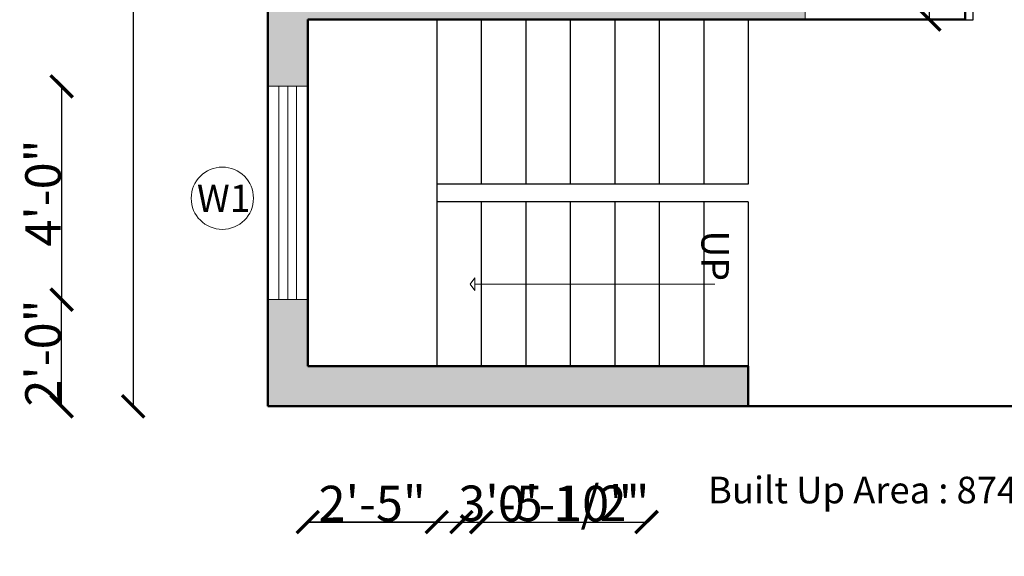
# Model space of a CAD drawing. Units: inches. Extents: x 1938 to 2373, y 1634 to 2225.
# Tile 1 of 5: x 1944 to 2166, y 1634 to 1755. Entities that reach past the tile are written whole.
import ezdxf

# ---------------------------------------------------------------- set-up
doc = ezdxf.new("R2010")
doc.units = ezdxf.units.IN
for name, color, linetype, lineweight in [('A-ANNO-DIMS', 2, 'Continuous', 18), ('A-ANNO-SYMB', 7, 'Continuous', 18), ('A-ANNO-TEXT', 7, 'Continuous', 18), ('A-WALL-PATT', 82, 'Continuous', 13), ('MAIN DOOR', 150, 'Continuous', 25), ('STEPS', 50, 'Continuous', 25), ('WALL', 7, 'Continuous', 50), ('WINDOW', 150, 'Continuous', 18)]:
    doc.layers.add(name, color=color, linetype=linetype, lineweight=lineweight)
doc.layers.add('A-Glaz', color=92, linetype='Continuous')
doc.styles.get("Standard").update_dxf_attribs({"font": 'arial.ttf'})
doc.dimstyles.get("Standard").update_dxf_attribs({"dimtxt": 8, "dimasz": 5, "dimexe": 0.18, "dimexo": 0.0625, "dimgap": 0.09, "dimtad": 1, "dimdec": 1, "dimzin": 0, "dimdsep": 46, "dimlunit": 4, "dimtxsty": 'Standard', "dimblk": 'ARCHTICK', "dimcen": 0.09, "dimse1": 1, "dimse2": 1, "dimadec": 0, "dimazin": 0, "dimtfac": 1, "dimtdec": 1, "dimtofl": 0, "dimtmove": 0, "dimatfit": 3, "dimfxl": 1, "dimtolj": 1, "dimtzin": 0, "dimarcsym": 0})

# ---------------------------------------------------------------- blocks, each defined once
blk = doc.blocks.new('A$C13CE0A17')
at = {"layer": 'A-Glaz'}
for p, q in [((0.01, 0.61), (0.01, 0.08)), ((0.03, 0.08), (0.03, 0.61))]:
    blk.add_line(p, q, dxfattribs=at)
blk.add_lwpolyline([(1.4, 0.08), (1.4, 0.61), (1.42, 0.61), (1.42, 0.08)], close=True, dxfattribs=at)
at = {"layer": 'MAIN DOOR'}
for p, q in [((0, 0.61), (0, 0.69)), ((0, 0.69), (0.04, 0.69)), ((0.04, 0.69), (0.04, 0.61)), ((0, 0.61), (0, 0.08)), ((0.04, 0.61), (0, 0.61)), ((0.04, 0.61), (0, 0.61)), ((0.03, 0.61), (0.01, 0.61)), ((0.04, 0.08), (0.04, 0.61)), ((0, 0.08), (0, 0)), ((0.04, 0.08), (0, 0.08)), ((0, 0.08), (0.04, 0.08)), ((0.01, 0.08), (0.03, 0.08)), ((0.04, 0), (0.04, 0.08)), ((-0.035, 0), (-0.035, -0.1)), ((0, 0), (-0.035, 0)), ((0, 0), (0.04, 0)), ((0, -0.04), (0, 0)), ((0.015, -0.04), (0, -0.04)), ((0.015, -0.05), (0.015, -0.04)), ((0.015, -0.1), (0.015, -0.05)), ((-0.035, -0.1), (0.015, -0.1))]:
    blk.add_line(p, q, dxfattribs=at)
for points in [[(1.39, 0.69), (1.39, 0.61), (1.43, 0.61), (1.43, 0.69)], [(1.39, 0.08), (1.39, 0.61), (1.43, 0.61), (1.43, 0.08)], [(1.39, 0), (1.39, 0.08), (1.43, 0.08), (1.43, 0)], [(1.43, 0), (1.465, 0), (1.465, -0.1), (1.415, -0.1), (1.415, -0.05), (1.415, -0.04), (1.43, -0.04)]]:
    blk.add_lwpolyline(points, close=True, dxfattribs=at)
blk.add_arc((1.3872, 0.017), 0.673, 89.76573, 181.44381, dxfattribs=at)
blk.add_ellipse((0.0389, 0.0511), major_axis=(0.6669, -0.1217), ratio=0.940794, start_param=0.11153, end_param=1.73917, dxfattribs=at)
blk = doc.blocks.new('_ArchTick')
at = {"color": 0, "linetype": 'ByBlock', "const_width": 0.15}
blk.add_lwpolyline([(-0.5, -0.5), (0.5, 0.5)], dxfattribs=at)
blk = doc.blocks.new('*D13')
at = {"layer": 'A-ANNO-DIMS', "color": 0, "lineweight": -2, "transparency": 16777216}
blk.add_line((1969.98, 2123.59), (1969.98, 1667.59), dxfattribs=at)
at = {"layer": 'Defpoints', "color": 0, "transparency": 16777216}
for p in [(2000.23, 2123.59), (1969.98, 1667.59), (2000.23, 1667.59)]:
    blk.add_point(p, dxfattribs=at)
at = {"layer": 'A-ANNO-DIMS', "color": 0, "lineweight": -2, "transparency": 16777216, "xscale": 5, "yscale": 5, "zscale": 5}
for p, rotation in [((1969.98, 2123.59), 90), ((1969.98, 1667.59), 270)]:
    blk.add_blockref('_ArchTick', p, dxfattribs=dict(at, rotation=rotation))
at = {"layer": 'A-ANNO-DIMS', "color": 0, "transparency": 16777216, "insert": (1965.8, 1895.59), "char_height": 8, "attachment_point": 5, "rotation": 90}
blk.add_mtext("\\A1;38'", dxfattribs=at)
blk = doc.blocks.new('WIN-36IN-SIDELIGHT')
for p, q in [((36, 6.5), (0, 6.5)), ((36, 4.5), (0, 4.5)), ((36, 2.5), (0, 2.5))]:
    blk.add_line(p, q)
blk.add_lwpolyline([(36, 0), (36, 9), (0, 9), (0, 0)], close=True)
blk = doc.blocks.new('*D31')
at = {"layer": 'A-ANNO-DIMS', "color": 0, "lineweight": -2, "transparency": 16777216}
for p, q in [((2045.7, 1765.89), (2055.7, 1765.89)), ((2055.7, 1765.89), (2165.8, 1765.89))]:
    blk.add_line(p, q, dxfattribs=at)
at = {"layer": 'Defpoints', "color": 0, "transparency": 16777216}
for p in [(2045.7, 1767.39), (2055.7, 1767.39), (2055.7, 1765.89)]:
    blk.add_point(p, dxfattribs=at)
at = {"layer": 'A-ANNO-DIMS', "color": 0, "lineweight": -2, "transparency": 16777216, "xscale": 5, "yscale": 5, "zscale": 5, "rotation": 180}
blk.add_blockref('_ArchTick', (2045.7, 1765.89), dxfattribs=at)
at = {"layer": 'A-ANNO-DIMS', "color": 0, "lineweight": -2, "transparency": 16777216, "xscale": 5, "yscale": 5, "zscale": 5}
blk.add_blockref('_ArchTick', (2055.7, 1765.89), dxfattribs=at)
at = {"layer": 'A-ANNO-DIMS', "color": 0, "transparency": 16777216, "insert": (2113.25, 1770.06), "char_height": 8, "attachment_point": 5}
blk.add_mtext('\\A1;BURNER 0\'-10" TYP.', dxfattribs=at)
blk = doc.blocks.new('*D46')
at = {"layer": 'A-ANNO-DIMS', "color": 0, "lineweight": -2, "transparency": 16777216}
for p, q in [((2148.98, 1782.85), (2148.98, 1828.07)), ((2148.98, 1754.59), (2148.98, 1782.85))]:
    blk.add_line(p, q, dxfattribs=at)
at = {"layer": 'Defpoints', "color": 0, "transparency": 16777216}
for p in [(2148.98, 1782.85), (2157.02, 1782.85), (2157.02, 1754.59)]:
    blk.add_point(p, dxfattribs=at)
at = {"layer": 'A-ANNO-DIMS', "color": 0, "lineweight": -2, "transparency": 16777216, "xscale": 5, "yscale": 5, "zscale": 5}
for p, rotation in [((2148.98, 1782.85), 90), ((2148.98, 1754.59), 270)]:
    blk.add_blockref('_ArchTick', p, dxfattribs=dict(at, rotation=rotation))
at = {"layer": 'A-ANNO-DIMS', "color": 0, "transparency": 16777216, "insert": (2144.75, 1807.96), "char_height": 8, "attachment_point": 5, "rotation": 90}
blk.add_mtext('\\A1;2\'-4 1/2"', dxfattribs=at)
blk = doc.blocks.new('*D53')
at = {"layer": 'A-ANNO-DIMS', "color": 0, "lineweight": -2, "transparency": 16777216}
blk.add_line((1953.9, 1739.59), (1953.9, 1691.59), dxfattribs=at)
at = {"layer": 'Defpoints', "color": 0, "transparency": 16777216}
for p in [(2000.23, 1739.59), (1953.9, 1691.59), (2000.23, 1691.59)]:
    blk.add_point(p, dxfattribs=at)
at = {"layer": 'A-ANNO-DIMS', "color": 0, "lineweight": -2, "transparency": 16777216, "xscale": 5, "yscale": 5, "zscale": 5}
for p, rotation in [((1953.9, 1739.59), 90), ((1953.9, 1691.59), 270)]:
    blk.add_blockref('_ArchTick', p, dxfattribs=dict(at, rotation=rotation))
at = {"layer": 'A-ANNO-DIMS', "color": 0, "transparency": 16777216, "insert": (1949.72, 1715.59), "char_height": 8, "attachment_point": 5, "rotation": 90}
blk.add_mtext('\\A1;4\'-0"', dxfattribs=at)
blk = doc.blocks.new('*D54')
at = {"layer": 'A-ANNO-DIMS', "color": 0, "lineweight": -2, "transparency": 16777216}
blk.add_line((1953.9, 1667.59), (1953.9, 1691.59), dxfattribs=at)
at = {"layer": 'Defpoints', "color": 0, "transparency": 16777216}
for p in [(1953.9, 1691.59), (2000.23, 1691.59), (2000.23, 1667.59)]:
    blk.add_point(p, dxfattribs=at)
at = {"layer": 'A-ANNO-DIMS', "color": 0, "lineweight": -2, "transparency": 16777216, "xscale": 5, "yscale": 5, "zscale": 5}
for p, rotation in [((1953.9, 1691.59), 90), ((1953.9, 1667.59), 270)]:
    blk.add_blockref('_ArchTick', p, dxfattribs=dict(at, rotation=rotation))
at = {"layer": 'A-ANNO-DIMS', "color": 0, "transparency": 16777216, "insert": (1949.72, 1679.59), "char_height": 8, "attachment_point": 5, "rotation": 90}
blk.add_mtext('\\A1;2\'-0"', dxfattribs=at)
blk = doc.blocks.new('*D55')
at = {"layer": 'A-ANNO-DIMS', "color": 0, "lineweight": -2, "transparency": 16777216}
for p, q in [((2038.23, 1641.54), (2048.23, 1641.54)), ((2048.23, 1641.54), (2080.89, 1641.54))]:
    blk.add_line(p, q, dxfattribs=at)
at = {"layer": 'Defpoints', "color": 0, "transparency": 16777216}
for p in [(2038.23, 1676.59), (2048.23, 1676.59), (2048.23, 1641.54)]:
    blk.add_point(p, dxfattribs=at)
at = {"layer": 'A-ANNO-DIMS', "color": 0, "lineweight": -2, "transparency": 16777216, "xscale": 5, "yscale": 5, "zscale": 5, "rotation": 180}
blk.add_blockref('_ArchTick', (2038.23, 1641.54), dxfattribs=at)
at = {"layer": 'A-ANNO-DIMS', "color": 0, "lineweight": -2, "transparency": 16777216, "xscale": 5, "yscale": 5, "zscale": 5}
blk.add_blockref('_ArchTick', (2048.23, 1641.54), dxfattribs=at)
at = {"layer": 'A-ANNO-DIMS', "color": 0, "transparency": 16777216, "insert": (2067.06, 1645.71), "char_height": 8, "attachment_point": 5}
blk.add_mtext('\\A1;0\'-10"', dxfattribs=at)
blk = doc.blocks.new('*D56')
at = {"layer": 'A-ANNO-DIMS', "color": 0, "lineweight": -2, "transparency": 16777216}
blk.add_line((2318.07, 1676.59), (2318.07, 1713.59), dxfattribs=at)
at = {"layer": 'Defpoints', "color": 0, "transparency": 16777216}
for p in [(2108.23, 1713.59), (2318.07, 1713.59), (2108.23, 1676.59)]:
    blk.add_point(p, dxfattribs=at)
at = {"layer": 'A-ANNO-DIMS', "color": 0, "lineweight": -2, "transparency": 16777216, "xscale": 5, "yscale": 5, "zscale": 5}
for p, rotation in [((2318.07, 1713.59), 90), ((2318.07, 1676.59), 270)]:
    blk.add_blockref('_ArchTick', p, dxfattribs=dict(at, rotation=rotation))
at = {"layer": 'A-ANNO-DIMS', "color": 0, "transparency": 16777216, "insert": (2313.89, 1695.09), "char_height": 8, "attachment_point": 5, "rotation": 90}
blk.add_mtext('\\A1;3\'-1"', dxfattribs=at)
blk = doc.blocks.new('*D57')
at = {"layer": 'A-ANNO-DIMS', "color": 0, "lineweight": -2, "transparency": 16777216}
blk.add_line((2009.23, 1641.54), (2038.23, 1641.54), dxfattribs=at)
at = {"layer": 'Defpoints', "color": 0, "transparency": 16777216}
for p in [(2009.23, 1676.59), (2038.23, 1676.59), (2038.23, 1641.54)]:
    blk.add_point(p, dxfattribs=at)
at = {"layer": 'A-ANNO-DIMS', "color": 0, "lineweight": -2, "transparency": 16777216, "xscale": 5, "yscale": 5, "zscale": 5, "rotation": 180}
blk.add_blockref('_ArchTick', (2009.23, 1641.54), dxfattribs=at)
at = {"layer": 'A-ANNO-DIMS', "color": 0, "lineweight": -2, "transparency": 16777216, "xscale": 5, "yscale": 5, "zscale": 5}
blk.add_blockref('_ArchTick', (2038.23, 1641.54), dxfattribs=at)
at = {"layer": 'A-ANNO-DIMS', "color": 0, "transparency": 16777216, "insert": (2023.73, 1645.71), "char_height": 8, "attachment_point": 5}
blk.add_mtext('\\A1;2\'-5"', dxfattribs=at)
blk = doc.blocks.new('*D67')
at = {"layer": 'A-ANNO-DIMS', "color": 0, "lineweight": -2, "transparency": 16777216}
blk.add_line((2038.23, 1641.54), (2009.23, 1641.54), dxfattribs=at)
at = {"layer": 'Defpoints', "color": 0, "transparency": 16777216}
for p in [(2038.23, 1792.59), (2009.23, 1763.59), (2009.23, 1641.54)]:
    blk.add_point(p, dxfattribs=at)
at = {"layer": 'A-ANNO-DIMS', "color": 0, "lineweight": -2, "transparency": 16777216, "xscale": 5, "yscale": 5, "zscale": 5, "rotation": 180}
blk.add_blockref('_ArchTick', (2009.23, 1641.54), dxfattribs=at)
at = {"layer": 'A-ANNO-DIMS', "color": 0, "lineweight": -2, "transparency": 16777216, "xscale": 5, "yscale": 5, "zscale": 5}
blk.add_blockref('_ArchTick', (2038.23, 1641.54), dxfattribs=at)
at = {"layer": 'A-ANNO-DIMS', "color": 0, "transparency": 16777216, "insert": (2023.73, 1645.71), "char_height": 8, "attachment_point": 5}
blk.add_mtext('\\A1;2\'-5"', dxfattribs=at)
blk = doc.blocks.new('*D69')
at = {"layer": 'A-ANNO-DIMS', "color": 0, "lineweight": -2, "transparency": 16777216}
blk.add_line((2043.75, 1641.54), (2085.39, 1641.54), dxfattribs=at)
at = {"layer": 'Defpoints', "color": 0, "transparency": 16777216}
for p in [(2043.75, 1765.79), (2085.39, 1765.79), (2085.39, 1641.54)]:
    blk.add_point(p, dxfattribs=at)
at = {"layer": 'A-ANNO-DIMS', "color": 0, "lineweight": -2, "transparency": 16777216, "xscale": 5, "yscale": 5, "zscale": 5, "rotation": 180}
blk.add_blockref('_ArchTick', (2043.75, 1641.54), dxfattribs=at)
at = {"layer": 'A-ANNO-DIMS', "color": 0, "lineweight": -2, "transparency": 16777216, "xscale": 5, "yscale": 5, "zscale": 5}
blk.add_blockref('_ArchTick', (2085.39, 1641.54), dxfattribs=at)
at = {"layer": 'A-ANNO-DIMS', "color": 0, "transparency": 16777216, "insert": (2064.57, 1645.76), "char_height": 8, "attachment_point": 5}
blk.add_mtext('\\A1;3\'-5 1/2"', dxfattribs=at)

msp = doc.modelspace()

# ---------------------------------------------------------------- hatches: boundary and pattern name
at = {"layer": 'A-ANNO-SYMB'}
h = msp.add_hatch(dxfattribs=at)
h.set_pattern_fill('ANGLE', color=256, angle=90)
h.set_pattern_definition([(90, (3746.884, -436.872), (-6.985, 4e-16), [5.08, -1.905]), (180, (3746.884, -436.872), (-9e-16, -6.985), [5.08, -1.905])])
h.paths.add_polyline_path([(2046.78, 1696.52), (2045.7, 1695.09), (2046.78, 1693.65)])
at = {"layer": 'A-WALL-PATT', "transparency": 33554585}
h = msp.add_hatch(color=256, dxfattribs=at)
h.dxf.hatch_style = 1
h.paths.add_polyline_path([(2076.23, 2123.59), (2000.23, 2123.59), (2000.23, 2078.59), (2009.23, 2078.59), (2009.23, 2078.85), (2009.23, 2114.59), (2076.23, 2114.59)])
h.paths.add_polyline_path([(2219.23, 2123.59), (2136.23, 2123.59), (2136.23, 2114.59), (2203.23, 2114.59), (2203.23, 2085.96), (2207.23, 2085.96), (2207.23, 2114.59), (2219.23, 2114.59)])
h.paths.add_polyline_path([(2276.23, 2123.59), (2255.23, 2123.59), (2255.23, 2114.59), (2262.62, 2114.59), (2267.23, 2114.59), (2267.23, 2050.59), (2203.23, 2050.59), (2203.23, 1978.59), (2207.23, 1978.59), (2207.23, 1984.65), (2207.23, 2046.59), (2267.23, 2046.59), (2267.23, 2032.59), (2276.23, 2032.59)])
h.paths.add_polyline_path([(2009.23, 2018.59), (2000.23, 2018.59), (2000.23, 1948.59), (2009.23, 1948.59), (2009.23, 1948.85), (2009.23, 1978.59), (2126.4, 1978.59), (2126.4, 1978.59), (2133.23, 1978.59), (2166.7, 1978.59), (2166.7, 1982.59), (2009.23, 1982.59)])
h.paths.add_polyline_path([(2276.23, 1996.59), (2267.23, 1996.59), (2267.23, 1982.59), (2237.23, 1982.59), (2237.23, 1978.59), (2267.23, 1978.59), (2267.23, 1901.32), (2276.23, 1901.32)])
h.paths.add_polyline_path([(2133.23, 1944.79), (2129.23, 1944.79), (2129.23, 1858.59), (2009.23, 1858.59), (2009.23, 1888.59), (2000.23, 1888.59), (2000.23, 1839.09), (2009.23, 1839.09), (2009.23, 1854.59), (2091.31, 1854.59), (2091.31, 1854.61), (2097.36, 1854.59), (2133.23, 1854.59)])
h.paths.add_polyline_path([(2121.02, 1763.59), (2097.23, 1763.59), (2097.23, 1824.61), (2093.23, 1824.61), (2093.23, 1763.59), (2009.23, 1763.59), (2009.23, 1779.09), (2000.23, 1779.09), (2000.23, 1739.59), (2009.23, 1739.59), (2009.23, 1754.59), (2121.02, 1754.59)])
h.paths.add_polyline_path([(2108.23, 1676.59), (2009.23, 1676.59), (2009.23, 1691.59), (2000.23, 1691.59), (2000.23, 1667.59), (2108.23, 1667.59)])
h.paths.add_polyline_path([(2276.23, 1841.32), (2267.23, 1841.32), (2267.23, 1763.59), (2246.64, 1763.59), (2246.64, 1754.59), (2276.23, 1754.59)])

# ---------------------------------------------------------------- linework, layer by layer
at = {"layer": 'A-ANNO-SYMB'}
for p, q in [((2045.7, 1695.09), (2046.78, 1696.52)), ((2046.78, 1693.65), (2046.78, 1696.52)), ((2045.7, 1695.09), (2046.78, 1693.65)), ((2100.77, 1695.09), (2046.78, 1695.09))]:
    msp.add_line(p, q, dxfattribs=at)
msp.add_circle((1990.03, 1714.41), 7, dxfattribs=at)
at = {"layer": 'STEPS'}
for p, q in [((2038.23, 1754.59), (2038.23, 1676.59)), ((2048.23, 1754.59), (2048.23, 1717.59)), ((2058.23, 1754.59), (2058.23, 1717.59)), ((2068.23, 1754.59), (2068.23, 1717.59)), ((2078.23, 1754.59), (2078.23, 1717.59)), ((2088.23, 1754.59), (2088.23, 1717.59)), ((2098.23, 1754.59), (2098.23, 1717.59)), ((2108.23, 1754.59), (2108.23, 1717.59)), ((2108.23, 1717.59), (2038.23, 1717.59)), ((2108.23, 1713.59), (2038.23, 1713.59)), ((2048.23, 1713.59), (2048.23, 1676.59)), ((2058.23, 1713.59), (2058.23, 1676.59)), ((2068.23, 1713.59), (2068.23, 1676.59)), ((2078.23, 1713.59), (2078.23, 1676.59)), ((2088.23, 1713.59), (2088.23, 1676.59)), ((2098.23, 1713.59), (2098.23, 1676.59)), ((2108.23, 1713.59), (2108.23, 1676.59))]:
    msp.add_line(p, q, dxfattribs=at)
at = {"layer": 'WALL'}
for p, q in [((2000.23, 2123.59), (2000.23, 1667.59)), ((2157.02, 1754.59), (2157.02, 1763.59)), ((2009.23, 1754.59), (2157.02, 1754.59)), ((2009.23, 1754.59), (2009.23, 1676.59)), ((2009.23, 1676.59), (2108.23, 1676.59)), ((2108.23, 1676.59), (2108.23, 1667.59)), ((2000.23, 1667.59), (2276.23, 1667.59))]:
    msp.add_line(p, q, dxfattribs=at)
at = {"layer": 'WINDOW'}
for p, q in [((2002.73, 1691.59), (2002.73, 1739.59)), ((2004.73, 1691.59), (2004.73, 1739.59)), ((2006.73, 1691.59), (2006.73, 1739.59))]:
    msp.add_line(p, q, dxfattribs=at)
msp.add_lwpolyline([(2000.23, 1691.59), (2009.23, 1691.59), (2009.23, 1739.59), (2000.23, 1739.59)], close=True, dxfattribs=at)

# ---------------------------------------------------------------- block references
at = {"layer": 'MAIN DOOR', "xscale": 35.74477478846772, "yscale": 35.74477478846772, "zscale": 35.74477478846772}
msp.add_blockref('A$C13CE0A17', (2158.27, 1758.16), dxfattribs=at)
at = {"layer": 'WINDOW'}
msp.add_blockref('WIN-36IN-SIDELIGHT', (2121.02, 1754.59), dxfattribs=at)

# ---------------------------------------------------------------- texts
at = {"layer": 'A-ANNO-SYMB'}
msp.add_text('W1', height=6.166, dxfattribs=at).set_placement((1984.31, 1711.31))
at = {"layer": 'A-ANNO-TEXT'}
msp.add_text('UP', height=6.166, rotation=270, dxfattribs=at).set_placement((2097.73, 1707.17))
at = {"layer": 'A-ANNO-TEXT', "insert": (2095.13, 1651.75), "char_height": 6, "attachment_point": 1}
msp.add_mtext_dynamic_manual_height_columns('\\pxqc;Built Up Area : 874.00 Sq. ft', width=110.651, gutter_width=30.83, heights=[0], dxfattribs=at)

# ---------------------------------------------------------------- dimensions: what is measured, and where the dimension line sits
at = {"layer": 'A-ANNO-DIMS'}
for base, p1, p2, override, picture, middle in [((1969.98, 1667.59), (2000.23, 2123.59), (2000.23, 1667.59), {"dimclrd": 0, "dimclre": 0, "dimclrt": 0}, '*D13', (1965.8, 1895.59)), ((2148.98, 1782.85), (2157.02, 1754.59), (2157.02, 1782.85), {"dimdec": 1, "dimlfac": 1, "dimrnd": 0, "dimzin": 1, "dimdsep": 46, "dimlunit": 4, "dimfrac": 2}, '*D46', (2144.75, 1807.96)), ((1953.9, 1691.59), (2000.23, 1739.59), (2000.23, 1691.59), {"dimdec": 1, "dimlfac": 1, "dimrnd": 0, "dimzin": 1, "dimdsep": 46, "dimlunit": 4, "dimfrac": 2}, '*D53', (1949.72, 1715.59)), ((2318.07, 1713.59), (2108.23, 1676.59), (2108.23, 1713.59), {"dimdec": 1, "dimlfac": 1, "dimrnd": 0, "dimzin": 1, "dimdsep": 46, "dimlunit": 4, "dimfrac": 2}, '*D56', (2313.89, 1695.09)), ((1953.9, 1691.59), (2000.23, 1667.59), (2000.23, 1691.59), {"dimdec": 1, "dimlfac": 1, "dimrnd": 0, "dimzin": 1, "dimdsep": 46, "dimlunit": 4, "dimfrac": 2}, '*D54', (1949.72, 1679.59))]:
    dim = msp.add_linear_dim(base=base, p1=p1, p2=p2, angle=90, dimstyle='Standard', override=override, dxfattribs=at)
    dim.commit()
    dim.dimension.update_dxf_attribs({"geometry": picture, "text_midpoint": middle})
for base, p1, p2, picture, middle in [((2009.23, 1641.54), (2038.23, 1792.59), (2009.23, 1763.59), '*D67', (2023.73, 1645.71)), ((2085.39, 1641.54), (2043.75, 1765.79), (2085.39, 1765.79), '*D69', (2064.57, 1645.76)), ((2038.23, 1641.54), (2009.23, 1676.59), (2038.23, 1676.59), '*D57', (2023.73, 1645.71)), ((2048.23, 1641.54), (2038.23, 1676.59), (2048.23, 1676.59), '*D55', (2067.06, 1645.71))]:
    dim = msp.add_linear_dim(base=base, p1=p1, p2=p2, dimstyle='Standard', override={"dimdec": 1, "dimlfac": 1, "dimrnd": 0, "dimzin": 1, "dimdsep": 46, "dimlunit": 4, "dimfrac": 2}, dxfattribs=at)
    dim.commit()
    dim.dimension.update_dxf_attribs({"geometry": picture, "text_midpoint": middle})
dim = msp.add_linear_dim(base=(2055.7, 1765.89), p1=(2045.7, 1767.39), p2=(2055.7, 1767.39), text='BURNER <> TYP.', dimstyle='Standard', override={"dimdec": 1, "dimlfac": 1, "dimrnd": 0, "dimzin": 1, "dimdsep": 46, "dimlunit": 4, "dimfrac": 2}, dxfattribs=at)
dim.commit()
dim.dimension.update_dxf_attribs({"geometry": '*D31', "text_midpoint": (2113.25, 1770.06)})

doc.saveas('drawing.dxf')
